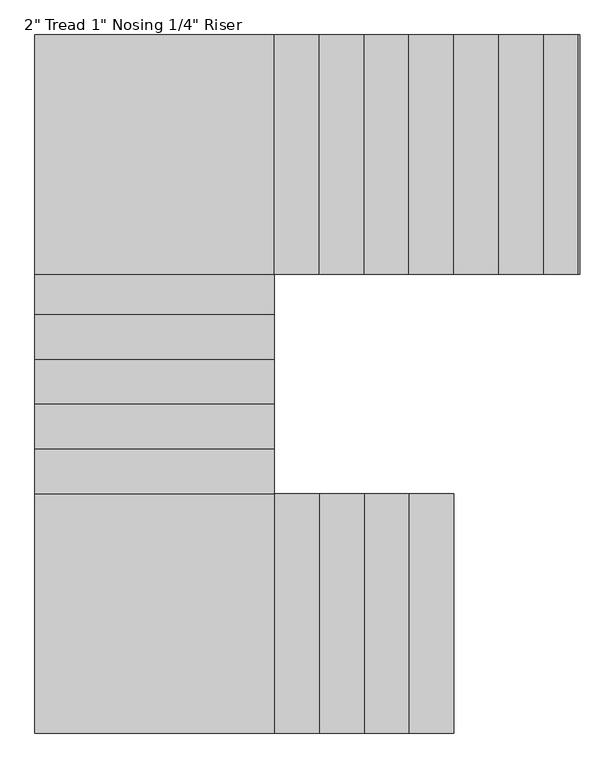
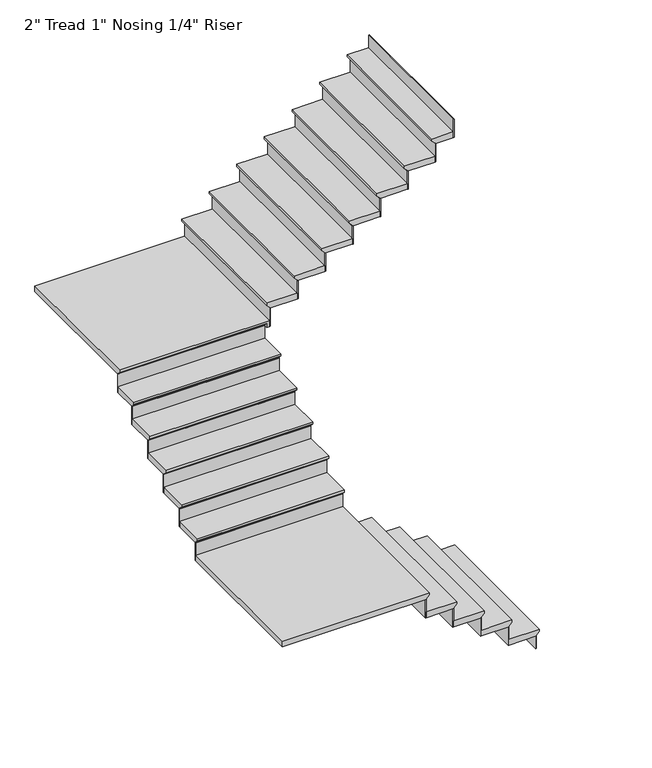
"""IFC4 building model written with IfcOpenShell, lengths in millimetres: stair flight geometry."""

from ifc_helpers import new_model, si_unit, origin, place, context, project, spatial, faceted_brep, source, transform, mapped, element, save


def stair_flight_f77ae209(model_context):
    return source(origin(), model_context, "Body", "Brep", [
        faceted_brep([(-2683.1105391, -1521.8373761, 19191.3710526), (-2683.1105391, -1521.8373761, 19210.4210526), (-2683.1105391, -2741.0373761, 19210.4210526), (-2683.1105391, -2741.0373761, 19191.3710526), (-2708.5105391, -1521.8373761, 19165.9710526), (-2708.5105391, -2741.0373761, 19165.9710526), (-2937.1105391, -1521.8373761, 19210.4210526), (-2937.1105391, -2741.0373761, 19210.4210526), (-2708.5105391, -2741.0373761, 19159.6210526), (-2937.1105391, -2741.0373761, 19159.6210526), (-2937.1105391, -1521.8373761, 19159.6210526), (-2708.5105391, -1521.8373761, 19159.6210526)], [[[0, 1, 2, 3]], [[4, 0, 3, 5]], [[2, 1, 6, 7]], [[8, 9, 10, 11]], [[2, 7, 9, 8, 5, 3]], [[8, 11, 4, 5]], [[6, 1, 0, 4, 11, 10]], [[7, 6, 10, 9]]]),
        faceted_brep([(-2708.5105391, -1521.8373761, 19159.6210526), (-2708.5105391, -1521.8373761, 19050.0), (-2714.8605391, -1521.8373761, 19050.0), (-2714.8605391, -1521.8373761, 19159.6210526), (-2708.5105391, -2741.0373761, 19159.6210526), (-2714.8605391, -2741.0373761, 19159.6210526), (-2714.8605391, -2741.0373761, 19050.0), (-2708.5105391, -2741.0373761, 19050.0)], [[[0, 1, 2, 3]], [[4, 5, 6, 7]], [[1, 0, 4, 7]], [[2, 1, 7, 6]], [[3, 2, 6, 5]], [[0, 3, 5, 4]]]),
        faceted_brep([(-2937.1105391, -1521.8373761, 19320.0421053), (-2937.1105391, -1521.8373761, 19159.6210526), (-2943.4605391, -1521.8373761, 19159.6210526), (-2943.4605391, -1521.8373761, 19320.0421053), (-2937.1105391, -2741.0373761, 19320.0421053), (-2943.4605391, -2741.0373761, 19320.0421053), (-2943.4605391, -2741.0373761, 19159.6210526), (-2937.1105391, -2741.0373761, 19159.6210526)], [[[0, 1, 2, 3]], [[4, 5, 6, 7]], [[1, 0, 4, 7]], [[2, 1, 7, 6]], [[3, 2, 6, 5]], [[0, 3, 5, 4]]]),
        faceted_brep([(-2911.7105391, -2741.0373761, 19370.8421053), (-2911.7105391, -1521.8373761, 19370.8421053), (-3165.7105391, -1521.8373761, 19370.8421053), (-3165.7105391, -2741.0373761, 19370.8421053), (-2937.1105391, -2741.0373761, 19320.0421053), (-3165.7105391, -2741.0373761, 19320.0421053), (-3165.7105391, -1521.8373761, 19320.0421053), (-2937.1105391, -1521.8373761, 19320.0421053), (-2937.1105391, -2741.0373761, 19326.3921053), (-2911.7105391, -2741.0373761, 19351.7921053), (-2937.1105391, -1521.8373761, 19326.3921053), (-2911.7105391, -1521.8373761, 19351.7921053)], [[[0, 1, 2, 3]], [[4, 5, 6, 7]], [[0, 3, 5, 4, 8, 9]], [[4, 7, 10, 8]], [[2, 1, 11, 10, 7, 6]], [[3, 2, 6, 5]], [[11, 1, 0, 9]], [[10, 11, 9, 8]]]),
        faceted_brep([(-3165.7105391, -1521.8373761, 19480.4631579), (-3165.7105391, -1521.8373761, 19320.0421053), (-3172.0605391, -1521.8373761, 19320.0421053), (-3172.0605391, -1521.8373761, 19480.4631579), (-3165.7105391, -2741.0373761, 19480.4631579), (-3172.0605391, -2741.0373761, 19480.4631579), (-3172.0605391, -2741.0373761, 19320.0421053), (-3165.7105391, -2741.0373761, 19320.0421053)], [[[0, 1, 2, 3]], [[4, 5, 6, 7]], [[1, 0, 4, 7]], [[2, 1, 7, 6]], [[3, 2, 6, 5]], [[0, 3, 5, 4]]]),
        faceted_brep([(-3140.3105391, -2741.0373761, 19531.2631579), (-3140.3105391, -1521.8373761, 19531.2631579), (-3394.3105391, -1521.8373761, 19531.2631579), (-3394.3105391, -2741.0373761, 19531.2631579), (-3165.7105391, -2741.0373761, 19480.4631579), (-3394.3105391, -2741.0373761, 19480.4631579), (-3394.3105391, -1521.8373761, 19480.4631579), (-3165.7105391, -1521.8373761, 19480.4631579), (-3165.7105391, -2741.0373761, 19486.8131579), (-3140.3105391, -2741.0373761, 19512.2131579), (-3165.7105391, -1521.8373761, 19486.8131579), (-3140.3105391, -1521.8373761, 19512.2131579)], [[[0, 1, 2, 3]], [[4, 5, 6, 7]], [[0, 3, 5, 4, 8, 9]], [[4, 7, 10, 8]], [[2, 1, 11, 10, 7, 6]], [[3, 2, 6, 5]], [[11, 1, 0, 9]], [[10, 11, 9, 8]]]),
        faceted_brep([(-3394.3105391, -1521.8373761, 19640.8842105), (-3394.3105391, -1521.8373761, 19480.4631579), (-3400.6605391, -1521.8373761, 19480.4631579), (-3400.6605391, -1521.8373761, 19640.8842105), (-3394.3105391, -2741.0373761, 19640.8842105), (-3400.6605391, -2741.0373761, 19640.8842105), (-3400.6605391, -2741.0373761, 19480.4631579), (-3394.3105391, -2741.0373761, 19480.4631579)], [[[0, 1, 2, 3]], [[4, 5, 6, 7]], [[1, 0, 4, 7]], [[2, 1, 7, 6]], [[3, 2, 6, 5]], [[0, 3, 5, 4]]]),
        faceted_brep([(-3368.9105391, -2741.0373761, 19691.6842105), (-3368.9105391, -1521.8373761, 19691.6842105), (-3622.9105391, -1521.8373761, 19691.6842105), (-3622.9105391, -2741.0373761, 19691.6842105), (-3394.3105391, -2741.0373761, 19640.8842105), (-3622.9105391, -2741.0373761, 19640.8842105), (-3622.9105391, -1521.8373761, 19640.8842105), (-3394.3105391, -1521.8373761, 19640.8842105), (-3394.3105391, -2741.0373761, 19647.2342105), (-3368.9105391, -2741.0373761, 19672.6342105), (-3394.3105391, -1521.8373761, 19647.2342105), (-3368.9105391, -1521.8373761, 19672.6342105)], [[[0, 1, 2, 3]], [[4, 5, 6, 7]], [[0, 3, 5, 4, 8, 9]], [[4, 7, 10, 8]], [[2, 1, 11, 10, 7, 6]], [[3, 2, 6, 5]], [[11, 1, 0, 9]], [[10, 11, 9, 8]]]),
        faceted_brep([(-3622.9105391, -1521.8373761, 19801.3052632), (-3622.9105391, -1521.8373761, 19640.8842105), (-3629.2605391, -1521.8373761, 19640.8842105), (-3629.2605391, -1521.8373761, 19801.3052632), (-3622.9105391, -2741.0373761, 19801.3052632), (-3629.2605391, -2741.0373761, 19801.3052632), (-3629.2605391, -2741.0373761, 19640.8842105), (-3622.9105391, -2741.0373761, 19640.8842105)], [[[0, 1, 2, 3]], [[4, 5, 6, 7]], [[1, 0, 4, 7]], [[2, 1, 7, 6]], [[3, 2, 6, 5]], [[0, 3, 5, 4]]]),
        faceted_brep([(-4816.7105391, -1496.4373761, 19852.1052632), (-4816.7105391, -2741.0373761, 19852.1052632), (-3597.5105391, -2741.0373761, 19852.1052632), (-3597.5105391, -1496.4373761, 19852.1052632), (-4816.7105391, -2741.0373761, 19801.3052632), (-4816.7105391, -1496.4373761, 19801.3052632), (-3597.5105391, -1496.4373761, 19801.3052632), (-3597.5105391, -1521.8373761, 19801.3052632), (-3622.9105391, -1521.8373761, 19801.3052632), (-3622.9105391, -2741.0373761, 19801.3052632), (-3622.9105391, -2741.0373761, 19807.6552632), (-3597.5105391, -2741.0373761, 19833.0552632), (-3622.9105391, -1521.8373761, 19807.6552632), (-3597.5105391, -1521.8373761, 19833.0552632)], [[[0, 1, 2, 3]], [[4, 5, 6, 7, 8, 9]], [[1, 0, 5, 4]], [[2, 1, 4, 9, 10, 11]], [[9, 8, 12, 10]], [[8, 7, 13, 12]], [[3, 2, 11, 13, 7, 6]], [[0, 3, 6, 5]], [[11, 10, 12, 13]]]),
        faceted_brep([(-3597.5105391, -1496.4373761, 19961.7263158), (-3597.5105391, -1496.4373761, 19801.3052632), (-3597.5105391, -1490.0873761, 19801.3052632), (-3597.5105391, -1490.0873761, 19961.7263158), (-4816.7105391, -1496.4373761, 19961.7263158), (-4816.7105391, -1490.0873761, 19961.7263158), (-4816.7105391, -1490.0873761, 19801.3052632), (-4816.7105391, -1496.4373761, 19801.3052632)], [[[0, 1, 2, 3]], [[4, 5, 6, 7]], [[1, 0, 4, 7]], [[2, 1, 7, 6]], [[3, 2, 6, 5]], [[0, 3, 5, 4]]]),
        faceted_brep([(-4816.7105391, -1521.8373761, 20012.5263158), (-3597.5105391, -1521.8373761, 20012.5263158), (-3597.5105391, -1267.8373761, 20012.5263158), (-4816.7105391, -1267.8373761, 20012.5263158), (-4816.7105391, -1496.4373761, 19961.7263158), (-4816.7105391, -1267.8373761, 19961.7263158), (-3597.5105391, -1267.8373761, 19961.7263158), (-3597.5105391, -1496.4373761, 19961.7263158), (-4816.7105391, -1496.4373761, 19968.0763158), (-4816.7105391, -1521.8373761, 19993.4763158), (-3597.5105391, -1496.4373761, 19968.0763158), (-3597.5105391, -1521.8373761, 19993.4763158)], [[[0, 1, 2, 3]], [[4, 5, 6, 7]], [[0, 3, 5, 4, 8, 9]], [[4, 7, 10, 8]], [[2, 1, 11, 10, 7, 6]], [[3, 2, 6, 5]], [[11, 1, 0, 9]], [[10, 11, 9, 8]]]),
        faceted_brep([(-3597.5105391, -1267.8373761, 20122.1473684), (-3597.5105391, -1267.8373761, 19961.7263158), (-3597.5105391, -1261.4873761, 19961.7263158), (-3597.5105391, -1261.4873761, 20122.1473684), (-4816.7105391, -1267.8373761, 20122.1473684), (-4816.7105391, -1261.4873761, 20122.1473684), (-4816.7105391, -1261.4873761, 19961.7263158), (-4816.7105391, -1267.8373761, 19961.7263158)], [[[0, 1, 2, 3]], [[4, 5, 6, 7]], [[1, 0, 4, 7]], [[2, 1, 7, 6]], [[3, 2, 6, 5]], [[0, 3, 5, 4]]]),
        faceted_brep([(-4816.7105391, -1293.2373761, 20172.9473684), (-3597.5105391, -1293.2373761, 20172.9473684), (-3597.5105391, -1039.2373761, 20172.9473684), (-4816.7105391, -1039.2373761, 20172.9473684), (-4816.7105391, -1267.8373761, 20122.1473684), (-4816.7105391, -1039.2373761, 20122.1473684), (-3597.5105391, -1039.2373761, 20122.1473684), (-3597.5105391, -1267.8373761, 20122.1473684), (-4816.7105391, -1267.8373761, 20128.4973684), (-4816.7105391, -1293.2373761, 20153.8973684), (-3597.5105391, -1267.8373761, 20128.4973684), (-3597.5105391, -1293.2373761, 20153.8973684)], [[[0, 1, 2, 3]], [[4, 5, 6, 7]], [[0, 3, 5, 4, 8, 9]], [[4, 7, 10, 8]], [[2, 1, 11, 10, 7, 6]], [[3, 2, 6, 5]], [[11, 1, 0, 9]], [[10, 11, 9, 8]]]),
        faceted_brep([(-3597.5105391, -1039.2373761, 20282.5684211), (-3597.5105391, -1039.2373761, 20122.1473684), (-3597.5105391, -1032.8873761, 20122.1473684), (-3597.5105391, -1032.8873761, 20282.5684211), (-4816.7105391, -1039.2373761, 20282.5684211), (-4816.7105391, -1032.8873761, 20282.5684211), (-4816.7105391, -1032.8873761, 20122.1473684), (-4816.7105391, -1039.2373761, 20122.1473684)], [[[0, 1, 2, 3]], [[4, 5, 6, 7]], [[1, 0, 4, 7]], [[2, 1, 7, 6]], [[3, 2, 6, 5]], [[0, 3, 5, 4]]]),
        faceted_brep([(-4816.7105391, -1064.6373761, 20333.3684211), (-3597.5105391, -1064.6373761, 20333.3684211), (-3597.5105391, -810.6373761, 20333.3684211), (-4816.7105391, -810.6373761, 20333.3684211), (-4816.7105391, -1039.2373761, 20282.5684211), (-4816.7105391, -810.6373761, 20282.5684211), (-3597.5105391, -810.6373761, 20282.5684211), (-3597.5105391, -1039.2373761, 20282.5684211), (-4816.7105391, -1039.2373761, 20288.9184211), (-4816.7105391, -1064.6373761, 20314.3184211), (-3597.5105391, -1039.2373761, 20288.9184211), (-3597.5105391, -1064.6373761, 20314.3184211)], [[[0, 1, 2, 3]], [[4, 5, 6, 7]], [[0, 3, 5, 4, 8, 9]], [[4, 7, 10, 8]], [[2, 1, 11, 10, 7, 6]], [[3, 2, 6, 5]], [[11, 1, 0, 9]], [[10, 11, 9, 8]]]),
        faceted_brep([(-3597.5105391, -810.6373761, 20442.9894737), (-3597.5105391, -810.6373761, 20282.5684211), (-3597.5105391, -804.2873761, 20282.5684211), (-3597.5105391, -804.2873761, 20442.9894737), (-4816.7105391, -810.6373761, 20442.9894737), (-4816.7105391, -804.2873761, 20442.9894737), (-4816.7105391, -804.2873761, 20282.5684211), (-4816.7105391, -810.6373761, 20282.5684211)], [[[0, 1, 2, 3]], [[4, 5, 6, 7]], [[1, 0, 4, 7]], [[2, 1, 7, 6]], [[3, 2, 6, 5]], [[0, 3, 5, 4]]]),
        faceted_brep([(-4816.7105391, -836.0373761, 20493.7894737), (-3597.5105391, -836.0373761, 20493.7894737), (-3597.5105391, -582.0373761, 20493.7894737), (-4816.7105391, -582.0373761, 20493.7894737), (-4816.7105391, -810.6373761, 20442.9894737), (-4816.7105391, -582.0373761, 20442.9894737), (-3597.5105391, -582.0373761, 20442.9894737), (-3597.5105391, -810.6373761, 20442.9894737), (-4816.7105391, -810.6373761, 20449.3394737), (-4816.7105391, -836.0373761, 20474.7394737), (-3597.5105391, -810.6373761, 20449.3394737), (-3597.5105391, -836.0373761, 20474.7394737)], [[[0, 1, 2, 3]], [[4, 5, 6, 7]], [[0, 3, 5, 4, 8, 9]], [[4, 7, 10, 8]], [[2, 1, 11, 10, 7, 6]], [[3, 2, 6, 5]], [[11, 1, 0, 9]], [[10, 11, 9, 8]]]),
        faceted_brep([(-3597.5105391, -582.0373761, 20603.4105263), (-3597.5105391, -582.0373761, 20442.9894737), (-3597.5105391, -575.6873761, 20442.9894737), (-3597.5105391, -575.6873761, 20603.4105263), (-4816.7105391, -582.0373761, 20603.4105263), (-4816.7105391, -575.6873761, 20603.4105263), (-4816.7105391, -575.6873761, 20442.9894737), (-4816.7105391, -582.0373761, 20442.9894737)], [[[0, 1, 2, 3]], [[4, 5, 6, 7]], [[1, 0, 4, 7]], [[2, 1, 7, 6]], [[3, 2, 6, 5]], [[0, 3, 5, 4]]]),
        faceted_brep([(-4816.7105391, -607.4373761, 20654.2105263), (-3597.5105391, -607.4373761, 20654.2105263), (-3597.5105391, -378.8373761, 20654.2105263), (-4816.7105391, -378.8373761, 20654.2105263), (-4816.7105391, -582.0373761, 20603.4105263), (-4816.7105391, -378.8373761, 20603.4105263), (-3597.5105391, -378.8373761, 20603.4105263), (-3597.5105391, -582.0373761, 20603.4105263), (-4816.7105391, -582.0373761, 20609.7605263), (-4816.7105391, -607.4373761, 20635.1605263), (-3597.5105391, -582.0373761, 20609.7605263), (-3597.5105391, -607.4373761, 20635.1605263)], [[[0, 1, 2, 3]], [[4, 5, 6, 7]], [[0, 3, 5, 4, 8, 9]], [[4, 7, 10, 8]], [[2, 1, 11, 10, 7, 6]], [[3, 2, 6, 5]], [[11, 1, 0, 9]], [[10, 11, 9, 8]]]),
        faceted_brep([(-3597.5105391, -378.8373761, 20763.8315789), (-3597.5105391, -378.8373761, 20603.4105263), (-3597.5105391, -372.4873761, 20603.4105263), (-3597.5105391, -372.4873761, 20763.8315789), (-4816.7105391, -378.8373761, 20763.8315789), (-4816.7105391, -372.4873761, 20763.8315789), (-4816.7105391, -372.4873761, 20603.4105263), (-4816.7105391, -378.8373761, 20603.4105263)], [[[0, 1, 2, 3]], [[4, 5, 6, 7]], [[1, 0, 4, 7]], [[2, 1, 7, 6]], [[3, 2, 6, 5]], [[0, 3, 5, 4]]]),
        faceted_brep([(-3572.1105391, 814.9626239, 20814.6315789), (-4816.7105391, 814.9626239, 20814.6315789), (-4816.7105391, -404.2373761, 20814.6315789), (-3572.1105391, -404.2373761, 20814.6315789), (-4816.7105391, 814.9626239, 20763.8315789), (-3572.1105391, 814.9626239, 20763.8315789), (-3572.1105391, -404.2373761, 20763.8315789), (-3597.5105391, -404.2373761, 20763.8315789), (-3597.5105391, -378.8373761, 20763.8315789), (-4816.7105391, -378.8373761, 20763.8315789), (-4816.7105391, -378.8373761, 20770.1815789), (-4816.7105391, -404.2373761, 20795.5815789), (-3597.5105391, -378.8373761, 20770.1815789), (-3597.5105391, -404.2373761, 20795.5815789)], [[[0, 1, 2, 3]], [[4, 5, 6, 7, 8, 9]], [[1, 0, 5, 4]], [[2, 1, 4, 9, 10, 11]], [[9, 8, 12, 10]], [[8, 7, 13, 12]], [[3, 2, 11, 13, 7, 6]], [[0, 3, 6, 5]], [[11, 10, 12, 13]]]),
        faceted_brep([(-3572.1105391, -404.2373761, 20924.2526316), (-3572.1105391, -404.2373761, 20763.8315789), (-3565.7605391, -404.2373761, 20763.8315789), (-3565.7605391, -404.2373761, 20924.2526316), (-3572.1105391, 814.9626239, 20924.2526316), (-3565.7605391, 814.9626239, 20924.2526316), (-3565.7605391, 814.9626239, 20763.8315789), (-3572.1105391, 814.9626239, 20763.8315789)], [[[0, 1, 2, 3]], [[4, 5, 6, 7]], [[1, 0, 4, 7]], [[2, 1, 7, 6]], [[3, 2, 6, 5]], [[0, 3, 5, 4]]]),
        faceted_brep([(-3597.5105391, 814.9626239, 20975.0526316), (-3597.5105391, -404.2373761, 20975.0526316), (-3343.5105391, -404.2373761, 20975.0526316), (-3343.5105391, 814.9626239, 20975.0526316), (-3572.1105391, 814.9626239, 20924.2526316), (-3343.5105391, 814.9626239, 20924.2526316), (-3343.5105391, -404.2373761, 20924.2526316), (-3572.1105391, -404.2373761, 20924.2526316), (-3572.1105391, 814.9626239, 20930.6026316), (-3597.5105391, 814.9626239, 20956.0026316), (-3572.1105391, -404.2373761, 20930.6026316), (-3597.5105391, -404.2373761, 20956.0026316)], [[[0, 1, 2, 3]], [[4, 5, 6, 7]], [[0, 3, 5, 4, 8, 9]], [[4, 7, 10, 8]], [[2, 1, 11, 10, 7, 6]], [[3, 2, 6, 5]], [[11, 1, 0, 9]], [[10, 11, 9, 8]]]),
        faceted_brep([(-3343.5105391, -404.2373761, 21084.6736842), (-3343.5105391, -404.2373761, 20924.2526316), (-3337.1605391, -404.2373761, 20924.2526316), (-3337.1605391, -404.2373761, 21084.6736842), (-3343.5105391, 814.9626239, 21084.6736842), (-3337.1605391, 814.9626239, 21084.6736842), (-3337.1605391, 814.9626239, 20924.2526316), (-3343.5105391, 814.9626239, 20924.2526316)], [[[0, 1, 2, 3]], [[4, 5, 6, 7]], [[1, 0, 4, 7]], [[2, 1, 7, 6]], [[3, 2, 6, 5]], [[0, 3, 5, 4]]]),
        faceted_brep([(-3368.9105391, 814.9626239, 21135.4736842), (-3368.9105391, -404.2373761, 21135.4736842), (-3114.9105391, -404.2373761, 21135.4736842), (-3114.9105391, 814.9626239, 21135.4736842), (-3343.5105391, 814.9626239, 21084.6736842), (-3114.9105391, 814.9626239, 21084.6736842), (-3114.9105391, -404.2373761, 21084.6736842), (-3343.5105391, -404.2373761, 21084.6736842), (-3343.5105391, 814.9626239, 21091.0236842), (-3368.9105391, 814.9626239, 21116.4236842), (-3343.5105391, -404.2373761, 21091.0236842), (-3368.9105391, -404.2373761, 21116.4236842)], [[[0, 1, 2, 3]], [[4, 5, 6, 7]], [[0, 3, 5, 4, 8, 9]], [[4, 7, 10, 8]], [[2, 1, 11, 10, 7, 6]], [[3, 2, 6, 5]], [[11, 1, 0, 9]], [[10, 11, 9, 8]]]),
        faceted_brep([(-3114.9105391, -404.2373761, 21245.0947368), (-3114.9105391, -404.2373761, 21084.6736842), (-3108.5605391, -404.2373761, 21084.6736842), (-3108.5605391, -404.2373761, 21245.0947368), (-3114.9105391, 814.9626239, 21245.0947368), (-3108.5605391, 814.9626239, 21245.0947368), (-3108.5605391, 814.9626239, 21084.6736842), (-3114.9105391, 814.9626239, 21084.6736842)], [[[0, 1, 2, 3]], [[4, 5, 6, 7]], [[1, 0, 4, 7]], [[2, 1, 7, 6]], [[3, 2, 6, 5]], [[0, 3, 5, 4]]]),
        faceted_brep([(-3140.3105391, 814.9626239, 21295.8947368), (-3140.3105391, -404.2373761, 21295.8947368), (-2886.3105391, -404.2373761, 21295.8947368), (-2886.3105391, 814.9626239, 21295.8947368), (-3114.9105391, 814.9626239, 21245.0947368), (-2886.3105391, 814.9626239, 21245.0947368), (-2886.3105391, -404.2373761, 21245.0947368), (-3114.9105391, -404.2373761, 21245.0947368), (-3114.9105391, 814.9626239, 21251.4447368), (-3140.3105391, 814.9626239, 21276.8447368), (-3114.9105391, -404.2373761, 21251.4447368), (-3140.3105391, -404.2373761, 21276.8447368)], [[[0, 1, 2, 3]], [[4, 5, 6, 7]], [[0, 3, 5, 4, 8, 9]], [[4, 7, 10, 8]], [[2, 1, 11, 10, 7, 6]], [[3, 2, 6, 5]], [[11, 1, 0, 9]], [[10, 11, 9, 8]]]),
        faceted_brep([(-2886.3105391, -404.2373761, 21405.5157895), (-2886.3105391, -404.2373761, 21245.0947368), (-2879.9605391, -404.2373761, 21245.0947368), (-2879.9605391, -404.2373761, 21405.5157895), (-2886.3105391, 814.9626239, 21405.5157895), (-2879.9605391, 814.9626239, 21405.5157895), (-2879.9605391, 814.9626239, 21245.0947368), (-2886.3105391, 814.9626239, 21245.0947368)], [[[0, 1, 2, 3]], [[4, 5, 6, 7]], [[1, 0, 4, 7]], [[2, 1, 7, 6]], [[3, 2, 6, 5]], [[0, 3, 5, 4]]]),
        faceted_brep([(-2911.7105391, 814.9626239, 21456.3157895), (-2911.7105391, -404.2373761, 21456.3157895), (-2657.7105391, -404.2373761, 21456.3157895), (-2657.7105391, 814.9626239, 21456.3157895), (-2886.3105391, 814.9626239, 21405.5157895), (-2657.7105391, 814.9626239, 21405.5157895), (-2657.7105391, -404.2373761, 21405.5157895), (-2886.3105391, -404.2373761, 21405.5157895), (-2886.3105391, 814.9626239, 21411.8657895), (-2911.7105391, 814.9626239, 21437.2657895), (-2886.3105391, -404.2373761, 21411.8657895), (-2911.7105391, -404.2373761, 21437.2657895)], [[[0, 1, 2, 3]], [[4, 5, 6, 7]], [[0, 3, 5, 4, 8, 9]], [[4, 7, 10, 8]], [[2, 1, 11, 10, 7, 6]], [[3, 2, 6, 5]], [[11, 1, 0, 9]], [[10, 11, 9, 8]]]),
        faceted_brep([(-2657.7105391, -404.2373761, 21565.9368421), (-2657.7105391, -404.2373761, 21405.5157895), (-2651.3605391, -404.2373761, 21405.5157895), (-2651.3605391, -404.2373761, 21565.9368421), (-2657.7105391, 814.9626239, 21565.9368421), (-2651.3605391, 814.9626239, 21565.9368421), (-2651.3605391, 814.9626239, 21405.5157895), (-2657.7105391, 814.9626239, 21405.5157895)], [[[0, 1, 2, 3]], [[4, 5, 6, 7]], [[1, 0, 4, 7]], [[2, 1, 7, 6]], [[3, 2, 6, 5]], [[0, 3, 5, 4]]]),
        faceted_brep([(-2683.1105391, 814.9626239, 21616.7368421), (-2683.1105391, -404.2373761, 21616.7368421), (-2429.1105391, -404.2373761, 21616.7368421), (-2429.1105391, 814.9626239, 21616.7368421), (-2657.7105391, 814.9626239, 21565.9368421), (-2429.1105391, 814.9626239, 21565.9368421), (-2429.1105391, -404.2373761, 21565.9368421), (-2657.7105391, -404.2373761, 21565.9368421), (-2657.7105391, 814.9626239, 21572.2868421), (-2683.1105391, 814.9626239, 21597.6868421), (-2657.7105391, -404.2373761, 21572.2868421), (-2683.1105391, -404.2373761, 21597.6868421)], [[[0, 1, 2, 3]], [[4, 5, 6, 7]], [[0, 3, 5, 4, 8, 9]], [[4, 7, 10, 8]], [[2, 1, 11, 10, 7, 6]], [[3, 2, 6, 5]], [[11, 1, 0, 9]], [[10, 11, 9, 8]]]),
        faceted_brep([(-2429.1105391, -404.2373761, 21726.3578947), (-2429.1105391, -404.2373761, 21565.9368421), (-2422.7605391, -404.2373761, 21565.9368421), (-2422.7605391, -404.2373761, 21726.3578947), (-2429.1105391, 814.9626239, 21726.3578947), (-2422.7605391, 814.9626239, 21726.3578947), (-2422.7605391, 814.9626239, 21565.9368421), (-2429.1105391, 814.9626239, 21565.9368421)], [[[0, 1, 2, 3]], [[4, 5, 6, 7]], [[1, 0, 4, 7]], [[2, 1, 7, 6]], [[3, 2, 6, 5]], [[0, 3, 5, 4]]]),
        faceted_brep([(-2454.5105391, 814.9626239, 21777.1578947), (-2454.5105391, -404.2373761, 21777.1578947), (-2200.5105391, -404.2373761, 21777.1578947), (-2200.5105391, 814.9626239, 21777.1578947), (-2429.1105391, 814.9626239, 21726.3578947), (-2200.5105391, 814.9626239, 21726.3578947), (-2200.5105391, -404.2373761, 21726.3578947), (-2429.1105391, -404.2373761, 21726.3578947), (-2429.1105391, 814.9626239, 21732.7078947), (-2454.5105391, 814.9626239, 21758.1078947), (-2429.1105391, -404.2373761, 21732.7078947), (-2454.5105391, -404.2373761, 21758.1078947)], [[[0, 1, 2, 3]], [[4, 5, 6, 7]], [[0, 3, 5, 4, 8, 9]], [[4, 7, 10, 8]], [[2, 1, 11, 10, 7, 6]], [[3, 2, 6, 5]], [[11, 1, 0, 9]], [[10, 11, 9, 8]]]),
        faceted_brep([(-2200.5105391, -404.2373761, 21886.7789474), (-2200.5105391, -404.2373761, 21726.3578947), (-2194.1605391, -404.2373761, 21726.3578947), (-2194.1605391, -404.2373761, 21886.7789474), (-2200.5105391, 814.9626239, 21886.7789474), (-2194.1605391, 814.9626239, 21886.7789474), (-2194.1605391, 814.9626239, 21726.3578947), (-2200.5105391, 814.9626239, 21726.3578947)], [[[0, 1, 2, 3]], [[4, 5, 6, 7]], [[1, 0, 4, 7]], [[2, 1, 7, 6]], [[3, 2, 6, 5]], [[0, 3, 5, 4]]]),
        faceted_brep([(-2048.1105391, -404.2373761, 22047.2), (-2048.1105391, -404.2373761, 21886.7789474), (-2041.7605391, -404.2373761, 21886.7789474), (-2041.7605391, -404.2373761, 22047.2), (-2048.1105391, 814.9626239, 22047.2), (-2041.7605391, 814.9626239, 22047.2), (-2041.7605391, 814.9626239, 21886.7789474), (-2048.1105391, 814.9626239, 21886.7789474)], [[[0, 1, 2, 3]], [[4, 5, 6, 7]], [[1, 0, 4, 7]], [[2, 1, 7, 6]], [[3, 2, 6, 5]], [[0, 3, 5, 4]]]),
        faceted_brep([(-2225.9105391, 814.9626239, 21937.5789474), (-2225.9105391, -404.2373761, 21937.5789474), (-2048.1105391, -404.2373761, 21937.5789474), (-2048.1105391, 814.9626239, 21937.5789474), (-2200.5105391, 814.9626239, 21886.7789474), (-2048.1105391, 814.9626239, 21886.7789474), (-2048.1105391, -404.2373761, 21886.7789474), (-2200.5105391, -404.2373761, 21886.7789474), (-2200.5105391, 814.9626239, 21893.1289474), (-2225.9105391, 814.9626239, 21918.5289474), (-2200.5105391, -404.2373761, 21893.1289474), (-2225.9105391, -404.2373761, 21918.5289474)], [[[0, 1, 2, 3]], [[4, 5, 6, 7]], [[0, 3, 5, 4, 8, 9]], [[4, 7, 10, 8]], [[2, 1, 11, 10, 7, 6]], [[3, 2, 6, 5]], [[11, 1, 0, 9]], [[10, 11, 9, 8]]]),
    ])


if __name__ == "__main__":
    model = new_model("IFC4")
    model_context = context("Model", 3, world=origin())
    ifc_project = project(units=[si_unit("LENGTHUNIT", "METRE", prefix="MILLI")], contexts=[model_context])
    site = spatial("IfcSite", under=ifc_project)
    building = spatial("IfcBuilding", under=site)
    placement = place(None, origin())
    stair_flight_shape = stair_flight_f77ae209(model_context)
    element("IfcStairFlight", 1, ObjectType="2\" Tread 1\" Nosing 1/4\" Riser", at=placement, inside=building, context=model_context, shape_type="MappedRepresentation", body=[
        mapped(stair_flight_shape, transform((0.0, 0.0, 0.0), x_axis=(1.0, 0.0, 0.0), y_axis=(0.0, 1.0, 0.0), z_axis=(0.0, 0.0, 1.0))),
    ])
    save(model, "model.ifc")
